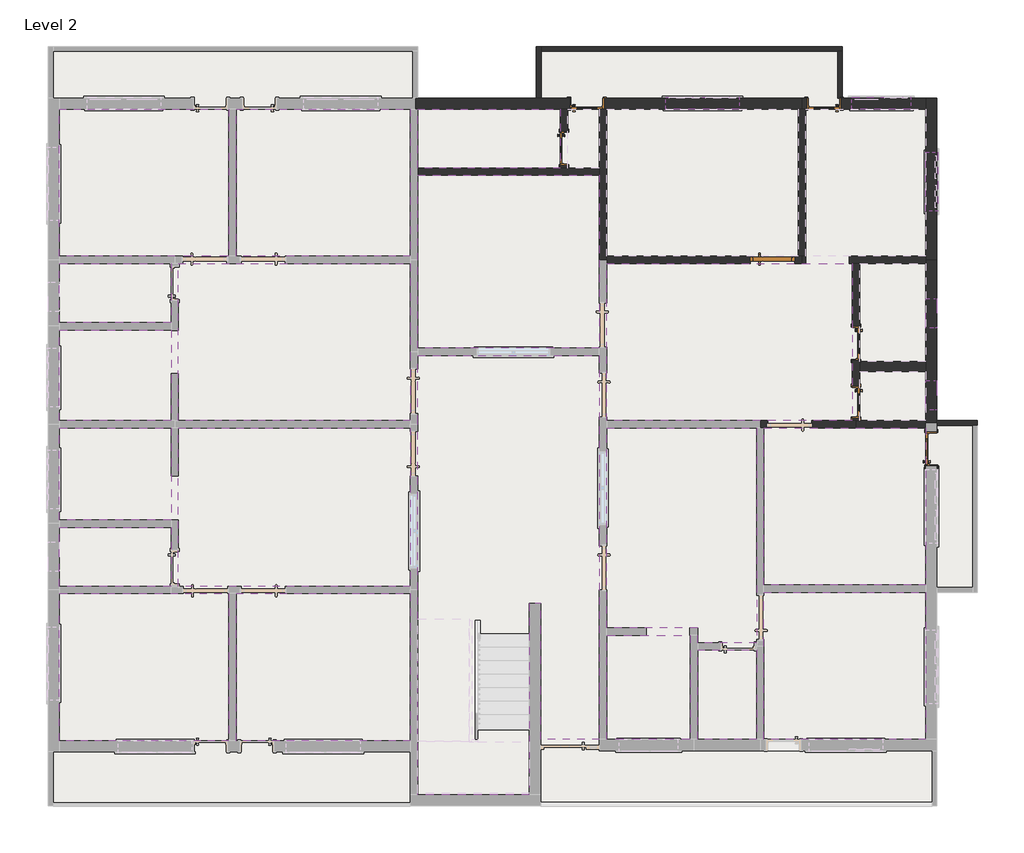
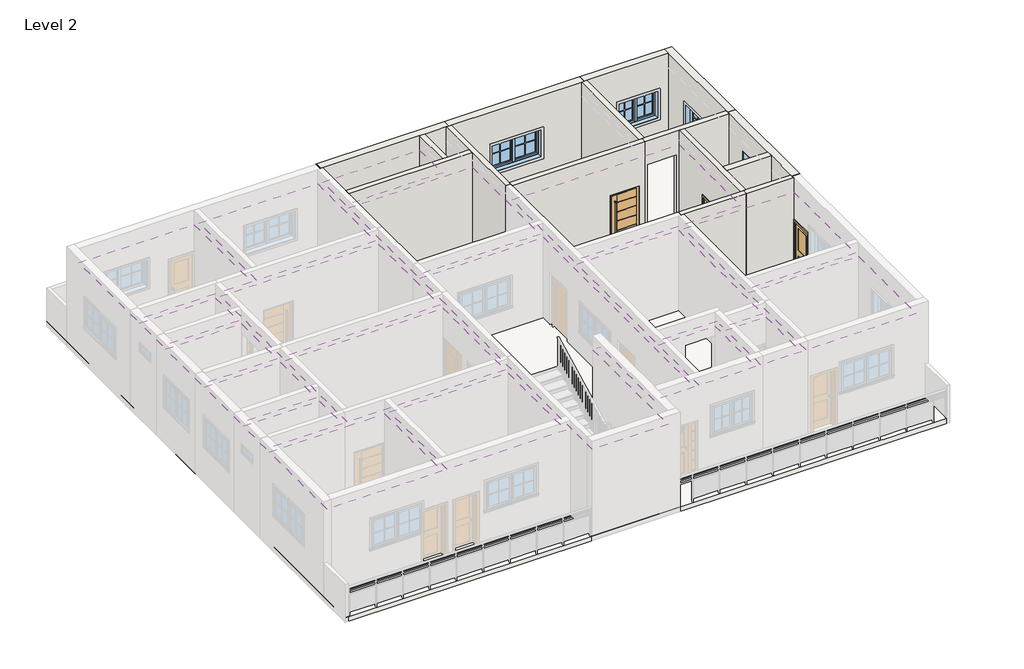
# One storey, part 3 of 5: 19 coverings, 19 walls, 7 doors, 5 windows, 1 slab.
# Revit data of these elements (continued)
# Materials (continued)
#   "Glass": class "Glass", colour RGB 0 128 192, transparency 0.75, Description = "Soda Lime Glass", Cost = 0
#   "Sash": class "Wood", colour RGB 224 178 126, transparency 0, Cost = 0
#   "Wood - Stained": class "Wood", colour RGB 224 178 126, transparency 0, Cost = 0
#   "Clad - White": class "Wood", colour RGB 242 242 238, transparency 0, Cost = 0
#   "Default Floor": colour RGB 128 128 128, transparency 0, Cost = 0
#   "OW1": class "Generic", colour RGB 120 120 120, transparency 0, Cost = 0
#   "FLT1": class "Generic", colour RGB 120 120 120, transparency 0, Cost = 0
#   "Default Wall": colour RGB 128 128 128, transparency 0, Cost = 0
#   "BRW1": class "Generic", colour RGB 120 120 120, transparency 0, Cost = 0
#   "LVW2": class "Generic", colour RGB 120 120 120, transparency 0, Cost = 0
#   "BRW2": class "Generic", colour RGB 120 120 120, transparency 0, Cost = 0
#   "BRW3": class "Generic", colour RGB 120 120 120, transparency 0, Cost = 0
#   "KW2": class "Generic", colour RGB 120 120 120, transparency 0, Cost = 0
